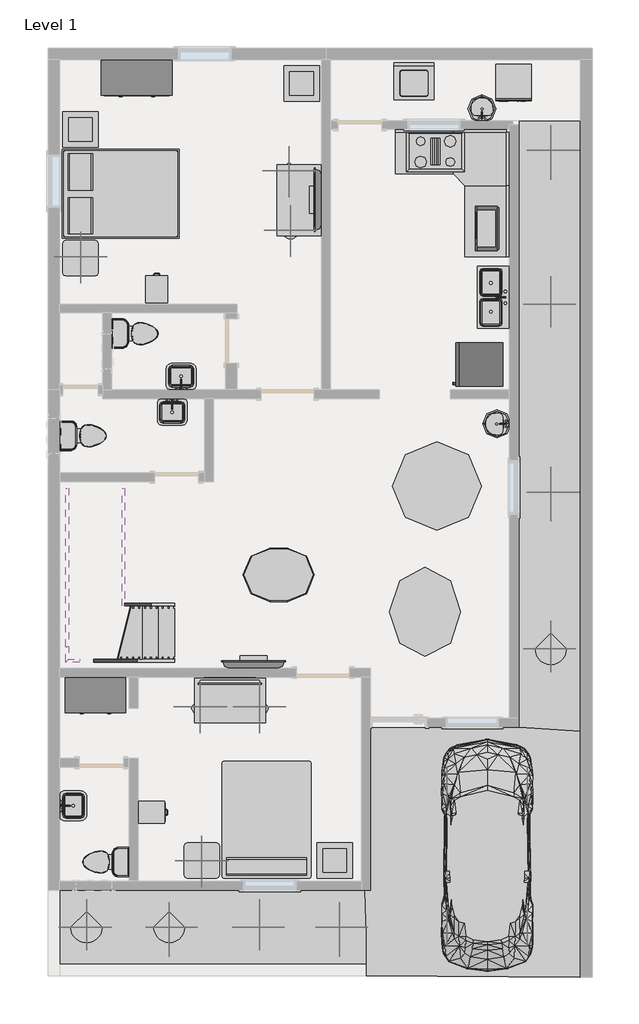
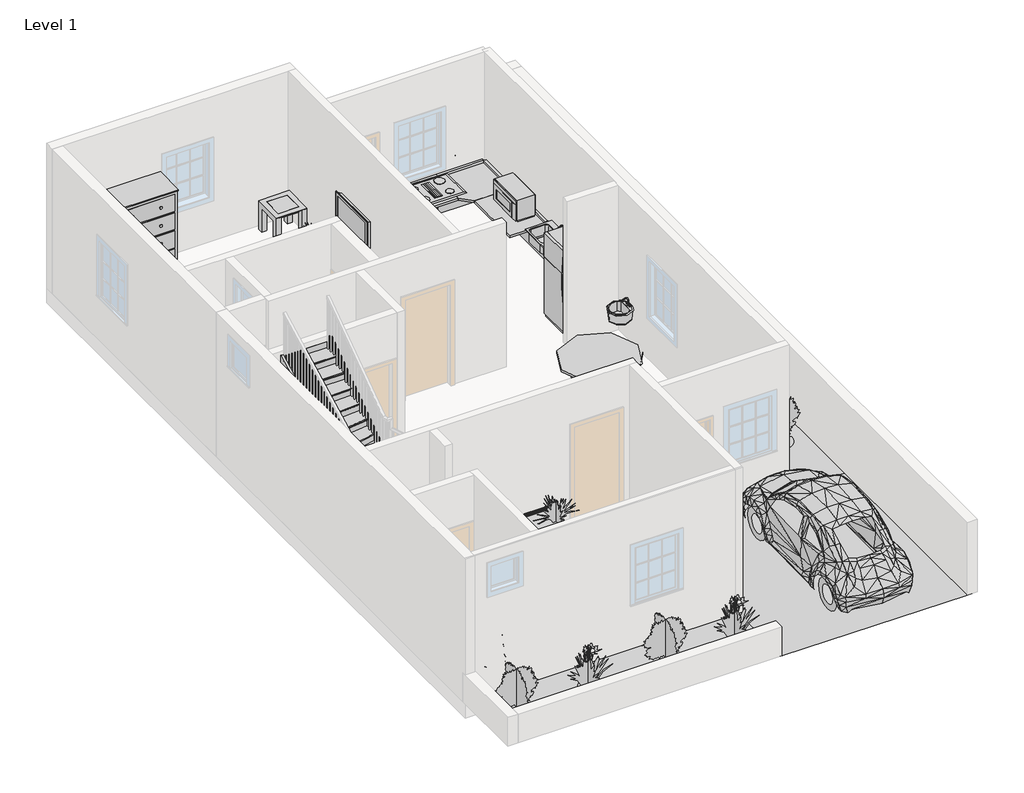
# One storey, part 3 of 3: 20 furniture elements, 14 geographic elements, 13 flow terminals, 9 proxies, 6 members, 1 stair flight.
"""IFC4 building model written with IfcOpenShell, lengths in millimetres."""

from ifc_helpers import new_model, si_unit, frame, origin, place, context, project, spatial, polyline, outline, extrude, triangles, transform, mapped, element, save
from components import proxy_bb1e6e30, proxy_45b28599, proxy_8a8d5ab2, rpc_beetle_rpc_beetle_3ce7ba48, proxy_a13a33b2, proxy_718fa39f, flow_terminal_accce45a, flow_terminal_a53be723, flow_terminal_d49f872f, flow_terminal_951b6bfb, flow_terminal_62a433f7, toilet_domestic_3d_toilet_domestic_3d_f7549cf7, toilet_domestic_3d_toilet_domestic_3d_183bbd19, furniture_1d2926bd, furniture_e1791683, furniture_bb55ed6b, furniture_9fa109b2, furniture_f72bdee3, furniture_7a3aaa4f, furniture_b5c51a22, furniture_be1c6672, furniture_bbcc68ce, furniture_743965d2, furniture_31d08a24, furniture_3f969c1c, furniture_5916b341, rpc_plant_tropical_55f6ff97, rpc_plant_tropical_agave_1_5_93a2a214, rpc_plant_tropical_jungle_flame_3_9c4808c2, stair_flight_28aaa101

model = new_model("IFC4")

# Units and contexts
model_context = context("Model", 3, world=origin())
ifc_project = project(units=[si_unit("LENGTHUNIT", "METRE", prefix="MILLI")], contexts=[model_context])

# Site, building, storey
site = spatial("IfcSite", under=ifc_project)
building = spatial("IfcBuilding", under=site)
storey = spatial("IfcBuildingStorey", under=building, Name="Level 1", Elevation=0.0)

# Proxies
placement = place(None, origin())
element("IfcBuildingElementProxy", 1, Name="Building Element Proxy", at=placement, inside=storey, context=model_context, shape_type="Tessellation", body=[
    triangles([(-6443.4660004, 13125.3534943, 0.0), (-5389.3658066, 13125.3534943, 0.0), (-5186.1660004, -971.6463604, 0.0), (-6433.8340302, -964.493018, 0.0)], [[1, 4, 2], [3, 2, 4]], closed=False),
])
element("IfcBuildingElementProxy", 2, Name="Building Element Proxy", at=placement, inside=storey, context=model_context, shape_type="Tessellation", body=[
    triangles([(-6443.4660004, 2711.353688, 0.0), (-9097.7661942, 2620.6554451, 0.0), (-9072.3660004, -147.5205558, 0.0), (-9096.8214844, -157.0514058, 0.0), (-9072.3660004, -1073.2463362, 0.0), (-6423.6154678, -976.648962, 0.0), (-9097.7661942, 2711.353688, 0.0), (-9072.3660004, -1555.846312, 0.0), (-5389.3658066, -1581.2463604, 0.0), (-5186.1660004, -1581.2463604, 0.0), (-5389.3658066, 2646.3030075, 0.0)], [[8, 5, 4], [5, 8, 6], [3, 2, 4], [7, 2, 1], [3, 4, 5], [6, 9, 10], [6, 3, 5], [6, 10, 11], [6, 1, 3], [1, 6, 11], [3, 1, 2], [6, 8, 9]], closed=False),
])
element("IfcBuildingElementProxy", 3, Name="Building Element Proxy", at=placement, inside=storey, context=model_context, shape_type="Tessellation", body=[
    triangles([(-14330.1660004, -82.6463725, 0.0), (-14330.1660004, -870.0463846, 0.0), (-9097.7661942, -82.6463725, 0.0), (-9072.3660004, -870.0463846, 0.0), (-14330.1660004, -1352.6463604, 0.0), (-9072.3660004, -1555.846312, 0.0)], [[4, 5, 6], [2, 5, 4], [1, 2, 3], [2, 4, 3]], closed=False),
])
proxy_shape = proxy_bb1e6e30(model_context)
element("IfcBuildingElementProxy", 4, Name="Cook Top-4 Unit : 36\" x 20\"", ObjectType="Cook Top-4 Unit : 36\" x 20\"", at=placement, inside=storey, context=model_context, shape_type="MappedRepresentation", body=[
    mapped(proxy_shape, transform((-7878.5660538, 12591.953629, 0.0), x_axis=(1.0, 0.0, 0.0), y_axis=(0.0, 1.0, 0.0), z_axis=(0.0, 0.0, 1.0))),
])
proxy_2_shape = proxy_45b28599(model_context)
element("IfcBuildingElementProxy", 5, Name="Dishwasher : 24\" x 24\" x 34\"", ObjectType="Dishwasher : 24\" x 24\" x 34\"", at=placement, inside=storey, context=model_context, shape_type="MappedRepresentation", body=[
    mapped(proxy_2_shape, transform((-6914.6835223, 13519.3040642, 0.0), x_axis=(1.0, 0.0, 0.0), y_axis=(0.0, 1.0, 0.0), z_axis=(0.0, 0.0, 1.0))),
])
proxy_3_shape = proxy_8a8d5ab2(model_context)
element("IfcBuildingElementProxy", 6, Name="Microwave : 30\" x 16\" x 18\"", ObjectType="Microwave : 30\" x 16\" x 18\"", at=placement, inside=storey, context=model_context, shape_type="MappedRepresentation", body=[
    mapped(proxy_3_shape, transform((-6636.485548, 11771.4465064, 0.0), x_axis=(0.0, -1.0000000000000007, 0.0), y_axis=(1.0000000000000007, 0.0, 0.0), z_axis=(0.0, 0.0, 1.0))),
])
rpc_beetle_rpc_beetle_shape = rpc_beetle_rpc_beetle_3ce7ba48(model_context)
element("IfcBuildingElementProxy", 7, Name="RPC Beetle : RPC Beetle", ObjectType="RPC Beetle : RPC Beetle", at=placement, inside=storey, context=model_context, shape_type="MappedRepresentation", body=[
    mapped(rpc_beetle_rpc_beetle_shape, transform((-6989.5660538, -717.646371, 0.0), x_axis=(1.0, 0.0, 0.0), y_axis=(0.0, 1.0, 0.0), z_axis=(0.0, 0.0, 1.0))),
])
proxy_4_shape = proxy_a13a33b2(model_context)
element("IfcBuildingElementProxy", 8, Name="Refrigerator : 30\" x 32\" RH", ObjectType="Refrigerator : 30\" x 32\" RH", at=placement, inside=storey, context=model_context, shape_type="MappedRepresentation", body=[
    mapped(proxy_4_shape, transform((-7109.0170823, 8942.291129, 0.0), x_axis=(0.0, -1.0000000000000007, 0.0), y_axis=(1.0000000000000007, 0.0, 0.0), z_axis=(0.0, 0.0, 1.0))),
])
proxy_5_shape = proxy_718fa39f(model_context)
element("IfcBuildingElementProxy", 9, Name="Washer : 27\" x 25\" x 35\"", ObjectType="Washer : 27\" x 25\" x 35\"", at=placement, inside=storey, context=model_context, shape_type="MappedRepresentation", body=[
    mapped(proxy_5_shape, transform((-8667.2835223, 13519.3040642, 0.0), x_axis=(1.0, 0.0, 0.0), y_axis=(0.0, 1.0, 0.0), z_axis=(0.0, 0.0, 1.0))),
])

# Flow terminals
flow_terminal_shape = flow_terminal_accce45a(model_context)
element("IfcFlowTerminal", 10, ObjectType="Floor Drain - Round : 5\" Strainer - 2\" Drain", at=placement, inside=storey, context=model_context, shape_type="MappedRepresentation", body=[
    mapped(flow_terminal_shape, transform((-13187.1660538, 8731.153629, 0.0), x_axis=(1.0, 0.0, 0.0), y_axis=(0.0, 1.0, 0.0), z_axis=(0.0, 0.0, 1.0))),
])
element("IfcFlowTerminal", 11, ObjectType="Floor Drain - Round : 5\" Strainer - 2\" Drain", at=placement, inside=storey, context=model_context, shape_type="MappedRepresentation", body=[
    mapped(flow_terminal_shape, transform((-13745.9660538, 7257.953629, 0.0), x_axis=(1.0, 0.0, 0.0), y_axis=(0.0, 1.0, 0.0), z_axis=(0.0, 0.0, 1.0))),
])
element("IfcFlowTerminal", 12, ObjectType="Floor Drain - Round : 5\" Strainer - 2\" Drain", at=placement, inside=storey, context=model_context, shape_type="MappedRepresentation", body=[
    mapped(flow_terminal_shape, transform((-14159.1367037, 774.6294473, 0.0), x_axis=(1.0, 0.0, 0.0), y_axis=(0.0, 1.0, 0.0), z_axis=(0.0, 0.0, 1.0))),
])
element("IfcFlowTerminal", 13, ObjectType="Floor Drain - Round : 5\" Strainer - 2\" Drain", at=placement, inside=storey, context=model_context, shape_type="MappedRepresentation", body=[
    mapped(flow_terminal_shape, transform((-7395.9660538, 13912.753629, 0.0), x_axis=(1.0, 0.0, 0.0), y_axis=(0.0, 1.0, 0.0), z_axis=(0.0, 0.0, 1.0))),
])
flow_terminal_2_shape = flow_terminal_a53be723(model_context)
element("IfcFlowTerminal", 14, ObjectType="Sink Kitchen-Double : 42\" x 21\"", at=placement, inside=storey, context=model_context, shape_type="MappedRepresentation", body=[
    mapped(flow_terminal_2_shape, transform((-6890.3114549, 10105.7428696, 0.0), x_axis=(0.0, -1.0000000000000002, 0.0), y_axis=(1.0000000000000002, 0.0, 0.0), z_axis=(0.0, 0.0, 1.0))),
])
flow_terminal_3_shape = flow_terminal_d49f872f(model_context)
element("IfcFlowTerminal", 15, ObjectType="Sink Vanity-Round : 19\" x 19\"", at=placement, inside=storey, context=model_context, shape_type="MappedRepresentation", body=[
    mapped(flow_terminal_3_shape, transform((-6981.8143133, 13408.8182168, 0.0), x_axis=(-1.0000000000000004, 0.0, 0.0), y_axis=(0.0, -1.0000000000000004, 0.0), z_axis=(0.0, 0.0, 1.0))),
])
flow_terminal_4_shape = flow_terminal_951b6bfb(model_context)
element("IfcFlowTerminal", 16, ObjectType="Sink Vanity-Round : 19\" x 19\"", at=placement, inside=storey, context=model_context, shape_type="MappedRepresentation", body=[
    mapped(flow_terminal_4_shape, transform((-6911.469597, 7821.7018885, 0.0), x_axis=(0.0, 1.0000000000000002, 0.0), y_axis=(-1.0000000000000002, 0.0, 0.0), z_axis=(0.0, 0.0, 1.0))),
])
flow_terminal_5_shape = flow_terminal_62a433f7(model_context)
element("IfcFlowTerminal", 17, ObjectType="Sink Vanity-Square : 20\" x 18\"", at=placement, inside=storey, context=model_context, shape_type="MappedRepresentation", body=[
    mapped(flow_terminal_5_shape, transform((-12231.6768133, 8682.6990301, 0.0), x_axis=(-1.0000000000000002, 0.0, 0.0), y_axis=(0.0, -1.0000000000000002, 0.0), z_axis=(0.0, 0.0, 1.0))),
])
element("IfcFlowTerminal", 18, ObjectType="Sink Vanity-Square : 20\" x 18\"", at=placement, inside=storey, context=model_context, shape_type="MappedRepresentation", body=[
    mapped(flow_terminal_5_shape, transform((-12415.4552944, 8170.0082279, 0.0), x_axis=(1.0, 0.0, 0.0), y_axis=(0.0, 1.0, 0.0), z_axis=(0.0, 0.0, 1.0))),
])
element("IfcFlowTerminal", 19, ObjectType="Sink Vanity-Square : 20\" x 18\"", at=placement, inside=storey, context=model_context, shape_type="MappedRepresentation", body=[
    mapped(flow_terminal_5_shape, transform((-14150.0206527, 1349.4643885, 0.0), x_axis=(0.0, 1.0000000000000002, 0.0), y_axis=(-1.0000000000000002, 0.0, 0.0), z_axis=(0.0, 0.0, 1.0))),
])
toilet_domestic_3d_toilet_domestic_3d_shape = toilet_domestic_3d_toilet_domestic_3d_f7549cf7(model_context)
toilet_domestic_3d_toilet_domestic_3d_2_shape = toilet_domestic_3d_toilet_domestic_3d_183bbd19(model_context)
element("IfcFlowTerminal", 20, ObjectType="Toilet-Domestic-3D : Toilet-Domestic-3D", at=placement, inside=storey, context=model_context, shape_type="MappedRepresentation", body=[
    mapped(toilet_domestic_3d_toilet_domestic_3d_shape, transform((-12946.4700265, 9467.753629, 0.0), x_axis=(0.0, 1.0, 0.0), y_axis=(-1.0, 0.0, 0.0), z_axis=(0.0, 0.0, 1.0))),
    mapped(toilet_domestic_3d_toilet_domestic_3d_2_shape, transform((-12946.4700265, 9467.753629, 0.0), x_axis=(0.0, 1.0, 0.0), y_axis=(-1.0, 0.0, 0.0), z_axis=(0.0, 0.0, 1.0))),
])
element("IfcFlowTerminal", 21, ObjectType="Toilet-Domestic-3D : Toilet-Domestic-3D", at=placement, inside=storey, context=model_context, shape_type="MappedRepresentation", body=[
    mapped(toilet_domestic_3d_toilet_domestic_3d_shape, transform((-13835.4700265, 7715.153629, 0.0), x_axis=(0.0, 1.0, 0.0), y_axis=(-1.0, 0.0, 0.0), z_axis=(0.0, 0.0, 1.0))),
    mapped(toilet_domestic_3d_toilet_domestic_3d_2_shape, transform((-13835.4700265, 7715.153629, 0.0), x_axis=(0.0, 1.0, 0.0), y_axis=(-1.0, 0.0, 0.0), z_axis=(0.0, 0.0, 1.0))),
])
element("IfcFlowTerminal", 22, ObjectType="Toilet-Domestic-3D : Toilet-Domestic-3D", at=placement, inside=storey, context=model_context, shape_type="MappedRepresentation", body=[
    mapped(toilet_domestic_3d_toilet_domestic_3d_shape, transform((-13631.0620812, 399.953629, 0.0), x_axis=(0.0, -1.0000000000000004, 0.0), y_axis=(1.0000000000000004, 0.0, 0.0), z_axis=(0.0, 0.0, 1.0))),
    mapped(toilet_domestic_3d_toilet_domestic_3d_2_shape, transform((-13631.0620812, 399.953629, 0.0), x_axis=(0.0, -1.0000000000000004, 0.0), y_axis=(1.0000000000000004, 0.0, 0.0), z_axis=(0.0, 0.0, 1.0))),
])

# Furniture
furniture_shape = furniture_1d2926bd(model_context)
element("IfcFurniture", 23, ObjectType="Bed-Box : Queen 60\" x 79\"", at=placement, inside=storey, context=model_context, shape_type="MappedRepresentation", body=[
    mapped(furniture_shape, transform((-13517.3660538, 11528.90117, 0.0), x_axis=(0.0, 1.0, 0.0), y_axis=(-1.0, 0.0, 0.0), z_axis=(0.0, 0.0, 1.0))),
])
furniture_2_shape = furniture_e1791683(model_context)
element("IfcFurniture", 24, ObjectType="Bed-Standard.0001 : Queen 60\" x 79\"", at=placement, inside=storey, context=model_context, shape_type="MappedRepresentation", body=[
    mapped(furniture_2_shape, transform((-10509.0275292, 1078.2585471, 0.0), x_axis=(-1.0, 0.0, 0.0), y_axis=(0.0, -1.0, 0.0), z_axis=(0.0, 0.0, 1.0))),
])
furniture_3_shape = furniture_bb55ed6b(model_context)
element("IfcFurniture", 25, ObjectType="Cabinet-File 2 Drawer : 15\" x 18\"", at=placement, inside=storey, context=model_context, shape_type="MappedRepresentation", body=[
    mapped(furniture_3_shape, transform((-12794.3625009, 10087.6193289, 0.0), x_axis=(-0.9999999999999999, 0.0, 0.0), y_axis=(0.0, -0.9999999999999999, 0.0), z_axis=(0.0, 0.0, 1.0))),
])
element("IfcFurniture", 26, ObjectType="Cabinet-File 2 Drawer : 15\" x 18\"", at=placement, inside=storey, context=model_context, shape_type="MappedRepresentation", body=[
    mapped(furniture_3_shape, transform((-12897.5003539, 1379.8516209, 0.0), x_axis=(0.0, 1.0, 0.0), y_axis=(-1.0, 0.0, 0.0), z_axis=(0.0, 0.0, 1.0))),
])
furniture_4_shape = furniture_9fa109b2(model_context)
element("IfcFurniture", 27, ObjectType="Dresser : 48\" x 72\" x 24\"", at=placement, inside=storey, context=model_context, shape_type="MappedRepresentation", body=[
    mapped(furniture_4_shape, transform((-12740.172794, 14225.1165831, 0.0), x_axis=(1.0, 0.0, 0.0), y_axis=(0.0, 1.0, 0.0), z_axis=(0.0, 0.0, 1.0))),
])
furniture_5_shape = furniture_f72bdee3(model_context)
element("IfcFurniture", 28, ObjectType="Dresser : 48\" x 72\" x 24\" 2", at=placement, inside=storey, context=model_context, shape_type="MappedRepresentation", body=[
    mapped(furniture_5_shape, transform((-13451.372794, 3633.3165831, 0.0), x_axis=(1.0, 0.0, 0.0), y_axis=(0.0, 1.0, 0.0), z_axis=(0.0, 0.0, 1.0))),
])
furniture_6_shape = furniture_7a3aaa4f(model_context)
element("IfcFurniture", 29, ObjectType="TV - Flat Screen : 42\"", at=placement, inside=storey, context=model_context, shape_type="MappedRepresentation", body=[
    mapped(furniture_6_shape, transform((-9892.9046775, 11762.5091149, 990.6), x_axis=(0.0, -1.0000000000000002, 0.0), y_axis=(1.0000000000000002, 0.0, 0.0), z_axis=(0.0, 0.0, 1.0))),
])
element("IfcFurniture", 30, ObjectType="TV - Flat Screen : 42\"", at=placement, inside=storey, context=model_context, shape_type="MappedRepresentation", body=[
    mapped(furniture_6_shape, transform((-11405.2215397, 3516.4150054, 0.0), x_axis=(1.0, 0.0, 0.0), y_axis=(0.0, 1.0, 0.0), z_axis=(0.0, 0.0, 1.0))),
])
element("IfcFurniture", 31, ObjectType="TV - Flat Screen : 42\"", at=placement, inside=storey, context=model_context, shape_type="MappedRepresentation", body=[
    mapped(furniture_6_shape, transform((-11006.710568, 3785.8922527, 990.6), x_axis=(-1.0000000000000002, 0.0, 0.0), y_axis=(0.0, -1.0000000000000002, 0.0), z_axis=(0.0, 0.0, 1.0))),
])
furniture_7_shape = furniture_b5c51a22(model_context)
element("IfcFurniture", 32, ObjectType="Table-Coffee : 24\" x 24\" x 24\"", at=placement, inside=storey, context=model_context, shape_type="MappedRepresentation", body=[
    mapped(furniture_7_shape, transform((-13992.8318205, 12877.7425512, 0.0), x_axis=(1.0, 0.0, 0.0), y_axis=(0.0, 1.0, 0.0), z_axis=(0.0, 0.0, 1.0))),
])
element("IfcFurniture", 33, ObjectType="Table-Coffee : 24\" x 24\" x 24\"", at=placement, inside=storey, context=model_context, shape_type="MappedRepresentation", body=[
    mapped(furniture_7_shape, transform((-10195.5318205, 13665.1425512, 0.0), x_axis=(1.0, 0.0, 0.0), y_axis=(0.0, 1.0, 0.0), z_axis=(0.0, 0.0, 1.0))),
])
element("IfcFurniture", 34, ObjectType="Table-Coffee : 24\" x 24\" x 24\"", at=placement, inside=storey, context=model_context, shape_type="MappedRepresentation", body=[
    mapped(furniture_7_shape, transform((-9624.0318205, 330.1425512, 0.0), x_axis=(1.0, 0.0, 0.0), y_axis=(0.0, 1.0, 0.0), z_axis=(0.0, 0.0, 1.0))),
])
furniture_8_shape = furniture_be1c6672(model_context)
element("IfcFurniture", 35, ObjectType="Table-Dining Oval : 36\" x 48\"", at=placement, inside=storey, context=model_context, shape_type="MappedRepresentation", body=[
    mapped(furniture_8_shape, transform((-10169.1463817, 5685.6519897, 0.0), x_axis=(1.0, 0.0, 0.0), y_axis=(0.0, 1.0, 0.0), z_axis=(0.0, 0.0, 1.0))),
])
furniture_9_shape = furniture_bbcc68ce(model_context)
element("IfcFurniture", 36, ObjectType="Table-Dining Round w Chairs : 60\" Diameter", at=placement, inside=storey, context=model_context, shape_type="MappedRepresentation", body=[
    mapped(furniture_9_shape, transform((-7956.848021, 7036.4323176, 0.0), x_axis=(1.0, 0.0, 0.0), y_axis=(0.0, 1.0, 0.0), z_axis=(0.0, 0.0, 1.0))),
])
furniture_10_shape = furniture_743965d2(model_context)
element("IfcFurniture", 37, ObjectType="Table-Ellipse : 60\" x 48\"", at=placement, inside=storey, context=model_context, shape_type="MappedRepresentation", body=[
    mapped(furniture_10_shape, transform((-8056.3660538, 4692.553629, 0.0), x_axis=(0.0, 1.0000000000000002, 0.0), y_axis=(-1.0000000000000002, 0.0, 0.0), z_axis=(0.0, 0.0, 1.0))),
])
furniture_11_shape = furniture_31d08a24(model_context)
element("IfcFurniture", 38, ObjectType="Table-End : 24\" x 24\"", at=placement, inside=storey, context=model_context, shape_type="MappedRepresentation", body=[
    mapped(furniture_11_shape, transform((-14283.0996841, 10610.753629, 0.0), x_axis=(1.0, 0.0, 0.0), y_axis=(0.0, 1.0, 0.0), z_axis=(0.0, 0.0, 1.0))),
])
element("IfcFurniture", 39, ObjectType="Table-End : 24\" x 24\"", at=placement, inside=storey, context=model_context, shape_type="MappedRepresentation", body=[
    mapped(furniture_11_shape, transform((-12200.2996841, 272.953629, 0.0), x_axis=(1.0, 0.0, 0.0), y_axis=(0.0, 1.0, 0.0), z_axis=(0.0, 0.0, 1.0))),
])
furniture_12_shape = furniture_3f969c1c(model_context)
element("IfcFurniture", 40, ObjectType="Table-Rectangular : 72\" x 30\"", at=placement, inside=storey, context=model_context, shape_type="MappedRepresentation", body=[
    mapped(furniture_12_shape, transform((-10215.3660538, 11753.753629, 0.0), x_axis=(0.0, 1.0000000000000002, 0.0), y_axis=(-1.0000000000000002, 0.0, 0.0), z_axis=(0.0, 0.0, 1.0))),
])
element("IfcFurniture", 41, ObjectType="Table-Rectangular : 72\" x 30\"", at=placement, inside=storey, context=model_context, shape_type="MappedRepresentation", body=[
    mapped(furniture_12_shape, transform((-11409.1660538, 3168.553629, 0.0), x_axis=(1.0, 0.0, 0.0), y_axis=(0.0, 1.0, 0.0), z_axis=(0.0, 0.0, 1.0))),
])
furniture_13_shape = furniture_5916b341(model_context)
element("IfcFurniture", 42, ObjectType="Work Station Cubicle : 96\" x 96\"", at=placement, inside=storey, context=model_context, shape_type="MappedRepresentation", body=[
    mapped(furniture_13_shape, transform((-6113.5430462, 12841.2218768, 0.0), x_axis=(0.0, -1.0000000000000004, 0.0), y_axis=(1.0000000000000004, 0.0, 0.0), z_axis=(0.0, 0.0, 1.0))),
])

# Geographic elements
rpc_plant_tropical_shape = rpc_plant_tropical_55f6ff97(model_context)
element("IfcGeographicElement", 43, ObjectType="RPC Plant - Tropical", at=placement, inside=storey, context=model_context, shape_type="MappedRepresentation", body=[
    mapped(rpc_plant_tropical_shape, transform((-5897.3660538, 12617.353629, 0.0), x_axis=(1.0, 0.0, 0.0), y_axis=(0.0, 1.0, 0.0), z_axis=(0.0, 0.0, 1.0))),
])
element("IfcGeographicElement", 44, ObjectType="RPC Plant - Tropical", at=placement, inside=storey, context=model_context, shape_type="MappedRepresentation", body=[
    mapped(rpc_plant_tropical_shape, transform((-5897.3660538, 6749.953629, 0.0), x_axis=(1.0, 0.0, 0.0), y_axis=(0.0, 1.0, 0.0), z_axis=(0.0, 0.0, 1.0))),
])
element("IfcGeographicElement", 45, ObjectType="RPC Plant - Tropical", at=placement, inside=storey, context=model_context, shape_type="MappedRepresentation", body=[
    mapped(rpc_plant_tropical_shape, transform((-12450.5660538, -717.646371, 0.0), x_axis=(1.0, 0.0, 0.0), y_axis=(0.0, 1.0, 0.0), z_axis=(0.0, 0.0, 1.0))),
])
element("IfcGeographicElement", 46, ObjectType="RPC Plant - Tropical", at=placement, inside=storey, context=model_context, shape_type="MappedRepresentation", body=[
    mapped(rpc_plant_tropical_shape, transform((-9529.5660538, -717.646371, 0.0), x_axis=(1.0, 0.0, 0.0), y_axis=(0.0, 1.0, 0.0), z_axis=(0.0, 0.0, 1.0))),
])
rpc_plant_tropical_agave_1_5_shape = rpc_plant_tropical_agave_1_5_93a2a214(model_context)
element("IfcGeographicElement", 47, ObjectType="RPC Plant - Tropical : Agave - 1.5'", at=placement, inside=storey, context=model_context, shape_type="MappedRepresentation", body=[
    mapped(rpc_plant_tropical_agave_1_5_shape, transform((-13974.5660538, 10788.553629, 609.6), x_axis=(1.0, 0.0, 0.0), y_axis=(0.0, 1.0, 0.0), z_axis=(0.0, 0.0, 1.0))),
])
element("IfcGeographicElement", 48, ObjectType="RPC Plant - Tropical : Agave - 1.5'", at=placement, inside=storey, context=model_context, shape_type="MappedRepresentation", body=[
    mapped(rpc_plant_tropical_agave_1_5_shape, transform((-10393.1660538, 12261.753629, 660.4), x_axis=(1.0, 0.0, 0.0), y_axis=(0.0, 1.0, 0.0), z_axis=(0.0, 0.0, 1.0))),
])
element("IfcGeographicElement", 49, ObjectType="RPC Plant - Tropical : Agave - 1.5'", at=placement, inside=storey, context=model_context, shape_type="MappedRepresentation", body=[
    mapped(rpc_plant_tropical_agave_1_5_shape, transform((-10367.7660538, 11245.753629, 660.4), x_axis=(1.0, 0.0, 0.0), y_axis=(0.0, 1.0, 0.0), z_axis=(0.0, 0.0, 1.0))),
])
element("IfcGeographicElement", 50, ObjectType="RPC Plant - Tropical : Agave - 1.5'", at=placement, inside=storey, context=model_context, shape_type="MappedRepresentation", body=[
    mapped(rpc_plant_tropical_agave_1_5_shape, transform((-11891.7660538, 425.353629, 609.6), x_axis=(1.0, 0.0, 0.0), y_axis=(0.0, 1.0, 0.0), z_axis=(0.0, 0.0, 1.0))),
])
element("IfcGeographicElement", 51, ObjectType="RPC Plant - Tropical : Agave - 1.5'", at=placement, inside=storey, context=model_context, shape_type="MappedRepresentation", body=[
    mapped(rpc_plant_tropical_agave_1_5_shape, transform((-11917.1660538, 3066.953629, 660.4), x_axis=(1.0, 0.0, 0.0), y_axis=(0.0, 1.0, 0.0), z_axis=(0.0, 0.0, 1.0))),
])
element("IfcGeographicElement", 52, ObjectType="RPC Plant - Tropical : Agave - 1.5'", at=placement, inside=storey, context=model_context, shape_type="MappedRepresentation", body=[
    mapped(rpc_plant_tropical_agave_1_5_shape, transform((-10901.1660538, 3066.953629, 660.4), x_axis=(1.0, 0.0, 0.0), y_axis=(0.0, 1.0, 0.0), z_axis=(0.0, 0.0, 1.0))),
])
rpc_plant_tropical_jungle_flame_3_shape = rpc_plant_tropical_jungle_flame_3_9c4808c2(model_context)
element("IfcGeographicElement", 53, ObjectType="RPC Plant - Tropical : Jungle Flame - 3'", at=placement, inside=storey, context=model_context, shape_type="MappedRepresentation", body=[
    mapped(rpc_plant_tropical_jungle_flame_3_shape, transform((-5897.3660538, 9975.753629, 0.0), x_axis=(1.0, 0.0, 0.0), y_axis=(0.0, 1.0, 0.0), z_axis=(0.0, 0.0, 1.0))),
])
element("IfcGeographicElement", 54, ObjectType="RPC Plant - Tropical : Jungle Flame - 3'", at=placement, inside=storey, context=model_context, shape_type="MappedRepresentation", body=[
    mapped(rpc_plant_tropical_jungle_flame_3_shape, transform((-5897.3660538, 4057.553629, 0.0), x_axis=(1.0, 0.0, 0.0), y_axis=(0.0, 1.0, 0.0), z_axis=(0.0, 0.0, 1.0))),
])
element("IfcGeographicElement", 55, ObjectType="RPC Plant - Tropical : Jungle Flame - 3'", at=placement, inside=storey, context=model_context, shape_type="MappedRepresentation", body=[
    mapped(rpc_plant_tropical_jungle_flame_3_shape, transform((-13872.9660538, -717.646371, 0.0), x_axis=(1.0, 0.0, 0.0), y_axis=(0.0, 1.0, 0.0), z_axis=(0.0, 0.0, 1.0))),
])
element("IfcGeographicElement", 56, ObjectType="RPC Plant - Tropical : Jungle Flame - 3'", at=placement, inside=storey, context=model_context, shape_type="MappedRepresentation", body=[
    mapped(rpc_plant_tropical_jungle_flame_3_shape, transform((-10901.1660538, -717.646371, 0.0), x_axis=(1.0, 0.0, 0.0), y_axis=(0.0, 1.0, 0.0), z_axis=(0.0, 0.0, 1.0))),
])

# Members
element("IfcMember", 57, ObjectType="Stringer - 2\" Width", at=placement, inside=storey, context=model_context, shape_type="SweptSolid", body=[
    extrude(outline(polyline([(590.0562463, -12359.4290643), (922.8849999, -12359.4290643), (1638.0971411, -13990.0912571), (1305.2683876, -13990.0912571), (590.0562463, -12359.4290643)])), frame((0.0, 3828.953629, 0.0), z_axis=(0.0, 1.0, 0.0), x_axis=(0.0, 0.0, 1.0)), (0.0, 0.0, 1.0), 50.8),
])
element("IfcMember", 58, ObjectType="Stringer - 2\" Width", at=placement, inside=storey, context=model_context, shape_type="SweptSolid", body=[
    extrude(outline(polyline([(-13990.0912571, 3879.753629), (-13990.0912571, 3828.953629), (-14228.5660538, 3828.953629), (-14177.7660538, 3879.753629), (-13990.0912571, 3879.753629)])), frame((0.0, 0.0, 1305.2683876), z_axis=(0.0, 0.0, 1.0), x_axis=(1.0, 0.0, 0.0)), (0.0, 0.0, 1.0), 332.8287535),
])
element("IfcMember", 59, ObjectType="Stringer - 2\" Width", at=placement, inside=storey, context=model_context, shape_type="SweptSolid", body=[
    extrude(outline(polyline([(-14177.7660538, 3879.753629), (-14228.5660538, 3828.953629), (-14228.5660538, 4097.9069721), (-14177.7660538, 4097.9069721), (-14177.7660538, 3879.753629)])), frame((0.0, 0.0, 1305.2683876), z_axis=(0.0, 0.0, 1.0), x_axis=(1.0, 0.0, 0.0)), (0.0, 0.0, 1.0), 332.8287535),
])
element("IfcMember", 60, ObjectType="Stringer - 2\" Width", at=placement, inside=storey, context=model_context, shape_type="SweptSolid", body=[
    extrude(outline(polyline([(4097.9069721, 1305.2683876), (4097.9069721, 1638.0971411), (6815.6906185, 3053.6189504), (6815.6906185, 2720.7901969), (4097.9069721, 1305.2683876)])), frame((-14228.5660538, 0.0, 0.0), z_axis=(1.0, 0.0, 0.0), x_axis=(0.0, 1.0, 0.0)), (0.0, 0.0, 1.0), 50.8),
])
element("IfcMember", 61, ObjectType="Stringer - 2\" Width", at=placement, inside=storey, context=model_context, shape_type="SweptSolid", body=[
    extrude(outline(polyline([(435.4922729, -12359.4290643), (842.634734, -12359.4290643), (1598.1690344, -13212.5660538), (1191.0265733, -13212.5660538), (435.4922729, -12359.4290643)])), frame((0.0, 4794.153629, 0.0), z_axis=(0.0, 1.0, 0.0), x_axis=(0.0, 0.0, 1.0)), (0.0, 0.0, 1.0), 50.8),
])
element("IfcMember", 62, ObjectType="Stringer - 2\" Width", at=placement, inside=storey, context=model_context, shape_type="SweptSolid", body=[
    extrude(outline(polyline([(4794.153629, 1337.7212805), (4794.153629, 1709.9296678), (6815.6906185, 3126.7693854), (6815.6906185, 2754.5609981), (4794.153629, 1337.7212805)])), frame((-13263.3660538, 0.0, 0.0), z_axis=(1.0, 0.0, 0.0), x_axis=(0.0, 1.0, 0.0)), (0.0, 0.0, 1.0), 50.8),
])

# Stair flight
stair_flight_shape = stair_flight_28aaa101(model_context)
element("IfcStairFlight", 63, ObjectType="2\" Tread 1\" Nosing 1/4\" Riser", at=placement, inside=storey, context=model_context, shape_type="MappedRepresentation", body=[
    mapped(stair_flight_shape, transform((0.0, 0.0, 0.0), x_axis=(1.0, 0.0, 0.0), y_axis=(0.0, 1.0, 0.0), z_axis=(0.0, 0.0, 1.0))),
])

save(model, "model.ifc")

# Revit data of these elements
# Type "Cook Top-4 Unit : 36\" x 20\""
#   Assembly Code = "E1090400"
#   Depth = 2' - 0"
#   Width = 3' - 0"
#   Burner Material = Steel, Chrome Plated
#   Cooktop Material = Steel, Polished
#   Default Elevation = 0
# Type "Dishwasher : 24\" x 24\" x 34\""
#   Label = "DW"
#   Assembly Code = "E1090400"
#   Depth = 2' - 0"
#   Height = 2' - 10"
#   Width = 2' - 0"
#   Dishwasher Material = Steel, Paint Finish, Ivory, Glossy
#   Panel Face Material = Plastic, Opaque Black
#   Default Elevation = 0
# Type "Microwave : 30\" x 16\" x 18\""
#   Assembly Code = "E1090400"
#   Depth = 1' - 4"
#   Height = 1' - 6"
#   Width = 2' - 6"
#   Microwave Material = Laminate, Ivory, Matte
#   Default Elevation = 0
# Type "RPC Beetle : RPC Beetle"
#   built-in parameter 1005195 = "RPC-16-0U6E-L4EG-ENH1-J3KF-SVEL-0TX4-C0"
#   Height = 0
# Type "Refrigerator : 30\" x 32\" RH"
#   Label = "REF."
#   Assembly Code = "E1090400"
#   Depth = 2' - 7 3/4"
#   Handle = 2' - 3"
#   Height = 5' - 10"
#   Rear Clearance = 0' - 2"
#   Top Door Height = 1' - 8"
#   Width = 2' - 5 3/8"
#   Material = Steel, Paint Finish, Ivory, Glossy
#   Default Elevation = 0
# Type "Washer : 27\" x 25\" x 35\""
#   Label = "W"
#   Assembly Code = "E1090400"
#   Depth = 2' - 1"
#   Height = 2' - 11"
#   Width = 2' - 3"
#   Washer Material = Steel, Paint Finish, Ivory, Matte
#   Default Elevation = 0
# Type "Floor Drain - Round : 5\" Strainer - 2\" Drain"
#   WFU = 2
#   Strainer Height = 0' - 3 1/4"
#   Strainer Radius = 0' - 2 1/2"
#   Strainer Diameter = 0' - 5"
#   Radius 6 = 0' - 0 5/8"
#   Radius 5 = 0' - 1 1/4"
#   Radius 4 = 0' - 1 7/8"
#   Radius 2 = 0' - 3.04167"
#   Radius 1 = 0' - 2.02083"
#   Radius 3 = 0' - 2 1/32"
#   Pipe Radius = 1"
#   Pipe Diameter = 2"
#   Height 2 = 0' - 0.725"
#   Height 1 = 0' - 1 13/16"
#   Body Radius = 0' - 4 1/16"
#   Body Height = 0' - 3 5/8"
#   Body Diameter = 0' - 8 1/8"
#   Drain Material = none
#   HWFU = 0
#   Default Elevation = 0
#   CWFU = 0
# Type "Sink Kitchen-Double : 42\" x 21\""
#   Assembly Code = "D2010410"
#   Counter Height = 3' - 0"
#   Depth = 1' - 9"
#   Width = 3' - 6"
#   Faucet Material = Steel, Polished
#   Sink Material = Steel, Polished
#   Default Elevation = 0
# Type "Sink Vanity-Round : 19\" x 19\""
#   Assembly Code = "D2010400"
#   Top Of Counter = 2' - 7"
#   Basin Material = Porcelain, Linen
#   Faucet Material = Steel, Polished
#   Default Elevation = 0
# Type "Sink Vanity-Square : 20\" x 18\""
#   Assembly Code = "D2010400"
#   Counter Height = 2' - 7"
#   Depth = 1' - 6"
#   Width = 1' - 8"
#   Basin Material = Porcelain, Linen
#   Faucet Material = Steel, Polished
#   Default Elevation = 0
# Type "Toilet-Domestic-3D : Toilet-Domestic-3D"
#   Assembly Code = "D2010110"
#   Toilet - Bowl/Basin Material = Porcelain, Linen
#   Toilet - Seat Material = Laminate, Linen, Matte
#   Default Elevation = 0
# Type "Bed-Box : Queen 60\" x 79\""
#   Assembly Code = "E2020200"
#   Length = 6' - 7"
#   Width = 5' - 0"
#   Frame Material = Birch
#   Mattress Material = Sash
#   Default Elevation = 0
# Type "Bed-Standard.0001 : Queen 60\" x 79\""
#   Assembly Code = "E2020200"
#   Length = 6' - 7"
#   Width = 5' - 0"
#   Leg Material = Steel, Chrome Plated
#   Mattress Material = Linen, White
#   Default Elevation = 0
# Type "Cabinet-File 2 Drawer : 15\" x 18\""
#   Assembly Code = "E2020200"
#   Depth = 1' - 6"
#   Height = 2' - 5"
#   Width = 1' - 3"
#   Cabinet Material = Steel, Paint Finish, Ivory, Glossy
#   Handle Material = Steel, Chrome Plated
#   Default Elevation = 0
# Type "Dresser : 48\" x 72\" x 24\""
#   Assembly Code = "E2020200"
#   Depth = 2' - 0"
#   Height = 6' - 0"
#   Width = 4' - 0"
#   Dresser Material = Wood - Teak
#   Drawer Material = Wood - Teak
#   Knob Material = Cherry
#   Default Elevation = 0
# Type "Dresser : 48\" x 72\" x 24\" 2"
#   Assembly Code = "E2020200"
#   Depth = 2' - 0"
#   Height = 6' - 0"
#   Width = 3' - 5"
#   Dresser Material = Wood - Teak
#   Drawer Material = Wood - Teak
#   Knob Material = Cherry
#   Default Elevation = 0
# Type "TV - Flat Screen : 42\""
#   SinAng = 0' - 0.0193"
#   L = 3' - 0.71517"
#   H = 1' - 8.65418"
#   Thickness = 0' - 4.33071"
#   Diagonal = 3' - 6.12598"
#   CosAng = 0' - 0.03431"
#   Stand [instance default] = yes
#   Default Elevation = 0
# Type "Table-Coffee : 24\" x 24\" x 24\""
#   Assembly Code = "E2020200"
#   Height = 2' - 0"
#   Length = 2' - 0"
#   Width = 2' - 0"
#   Top Material = none
#   Frame Material = none
#   Default Elevation = 0
# Type "Table-Dining Oval : 36\" x 48\""
#   Assembly Code = "E2020200"
#   Length = 4' - 0"
#   Width = 3' - 0"
#   Base Material = Steel, Chrome Plated
#   Top Material = Glass - Clear, Grey
#   Default Elevation = 0
#   Description = (empty or 0)
# Type "Table-Dining Round w Chairs : 60\" Diameter"
#   Assembly Code = "E2020200"
#   Radius = 2' - 6"
#   Diameter = 5' - 0"
#   Height = 2' - 6"
#   Chairs = 6
#   Base Material = Pine
#   Top Material = Laminate, Linen, Matte
#   Default Elevation = 0
# Type "Table-Ellipse : 60\" x 48\""
#   Assembly Code = "E2020200"
#   Half Width = 2' - 0"
#   Half Length = 2' - 6"
#   Height = 2' - 6"
#   Length = 5' - 0"
#   Width = 4' - 0"
#   Base Material = Birch
#   Top Material = Birch
#   Default Elevation = 0
# Type "Table-End : 24\" x 24\""
#   Assembly Code = "E2020200"
#   Height = 2' - 0"
#   Length = 2' - 0"
#   Width = 2' - 0"
#   Base Material = Birch
#   Top Material = Laminate, Ivory, Matte
#   Default Elevation = 0
# Type "Table-Rectangular : 72\" x 30\""
#   Assembly Code = "E2020200"
#   Height = 2' - 2"
#   Length = 4' - 0"
#   Width = 2' - 6"
#   Base Material = Birch
#   Top Material = Birch
#   Default Elevation = 0
# Type "Work Station Cubicle : 96\" x 96\""
#   Assembly Code = "E2020"
#   Desktop Height = 2' - 6"
#   Desktop1 Width = 2' - 4"
#   Desktop2 Width = 2' - 4"
#   Panel Height = 2' - 8"
#   Panel1 Length = 3' - 3"
#   Panel2 Length = 4' - 0"
#   Cube Panel Material = Textile - Light Gray
#   Work Top Material = Laminate, Ivory, Matte
#   Default Elevation = 0
# Type "RPC Plant - Tropical"
#   built-in parameter 1005198 = "{2, 15},{39, RPC-16-FWM5-GM7X-C67P-4000-ST1L-LVER-AU},{1, 0},{1, 0},{2, 13},{1, 8},{5, Color},{1, 0},{1, 0},{3, 0.8},{3, 0.8},{3, 0.8},{1, 8},{7, BBoxMin},{1, 0},{1, 0},{1, 0},{1, 0},{1, 0},{1, 8},{7, BBoxMax},{1, 0},{1, 0},{1, 0},{1, 0},{1, 0},{2, 11},{9, RPCTypeId},{1, 0},{1, 0},{39, RPC-16-FWM5-GM7X-C67P-4000-ST1L-LVER-AU},{1, 6},{14, RPCPlantHeight},{1, 0},{1, 0},{1, 3},{2, 11},{7, keyword},{1, 0},{1, 0},{35, :RPCs:Shrubs [General]:Geometry:RPC},{2, 11},{8, category},{1, 0},{1, 0},{16, Shrubs [General]},{2, 11},{12, LocalizedUID},{1, 0},{1, 0},{10, Crane Lily},{2, 14},{6, Height},{1, 0},{1, 0},{1, 3},{1, 2},{16, Cast Reflections},{1, 0},{1, 0},{1, 0},{1, 2},{12, Cast Shadows},{1, 0},{1, 0},{1, 1},{1, 2},{9, Lock View},{1, 0},{1, 0},{1, 0},{1, 4},{5, ViewC},{1, 0},{1, 0},{1, 0},{21, assetlibrary_base.fbx},{1, 5},"
#   built-in parameter 1005195 = "RPC-16-FWM5-GM7X-C67P-4000-ST1L-LVER-AU"
#   Assembly Code = "G2050500"
#   Height = 3' - 0"
#   Default Elevation = 0
# Type "RPC Plant - Tropical : Agave - 1.5'"
#   built-in parameter 1005198 = "{2, 15},{39, RPC-16-G1GJ-63FX-7K5P-N000-ST1L-LVER-AU},{1, 0},{1, 0},{2, 13},{1, 8},{5, Color},{1, 0},{1, 0},{3, 0.8},{3, 0.8},{3, 0.8},{1, 8},{7, BBoxMin},{1, 0},{1, 0},{1, 0},{1, 0},{1, 0},{1, 8},{7, BBoxMax},{1, 0},{1, 0},{1, 0},{1, 0},{1, 0},{2, 11},{9, RPCTypeId},{1, 0},{1, 0},{39, RPC-16-G1GJ-63FX-7K5P-N000-ST1L-LVER-AU},{1, 6},{14, RPCPlantHeight},{1, 0},{1, 0},{3, 1.5},{2, 11},{7, keyword},{1, 0},{1, 0},{35, :RPCs:Plants [General]:Geometry:RPC},{2, 11},{8, category},{1, 0},{1, 0},{16, Plants [General]},{2, 11},{12, LocalizedUID},{1, 0},{1, 0},{5, Agave},{2, 14},{6, Height},{1, 0},{1, 0},{3, 1.5},{1, 2},{16, Cast Reflections},{1, 0},{1, 0},{1, 0},{1, 2},{12, Cast Shadows},{1, 0},{1, 0},{1, 1},{1, 2},{9, Lock View},{1, 0},{1, 0},{1, 0},{1, 4},{5, ViewC},{1, 0},{1, 0},{1, 0},{21, assetlibrary_base.fbx},{1, 5},"
#   built-in parameter 1005195 = "RPC-16-G1GJ-63FX-7K5P-N000-ST1L-LVER-AU"
#   Type Comments = "Agave"
#   Assembly Code = "G2050500"
#   Height = 1' - 6"
#   Default Elevation = 0
# Type "RPC Plant - Tropical : Jungle Flame - 3'"
#   built-in parameter 1005198 = "{2, 15},{39, RPC-16-FUVJ-JWG0-MWGK-8000-ST1L-LVER-AU},{1, 0},{1, 0},{2, 13},{1, 8},{5, Color},{1, 0},{1, 0},{3, 0.8},{3, 0.8},{3, 0.8},{1, 8},{7, BBoxMin},{1, 0},{1, 0},{1, 0},{1, 0},{1, 0},{1, 8},{7, BBoxMax},{1, 0},{1, 0},{1, 0},{1, 0},{1, 0},{2, 11},{9, RPCTypeId},{1, 0},{1, 0},{39, RPC-16-FUVJ-JWG0-MWGK-8000-ST1L-LVER-AU},{1, 6},{14, RPCPlantHeight},{1, 0},{1, 0},{1, 3},{2, 11},{7, keyword},{1, 0},{1, 0},{35, :RPCs:Shrubs [General]:Geometry:RPC},{2, 11},{8, category},{1, 0},{1, 0},{16, Shrubs [General]},{2, 11},{12, LocalizedUID},{1, 0},{1, 0},{12, Jungle Flame},{2, 14},{6, Height},{1, 0},{1, 0},{1, 3},{1, 2},{16, Cast Reflections},{1, 0},{1, 0},{1, 0},{1, 2},{12, Cast Shadows},{1, 0},{1, 0},{1, 1},{1, 2},{9, Lock View},{1, 0},{1, 0},{1, 0},{1, 4},{5, ViewC},{1, 0},{1, 0},{1, 0},{21, assetlibrary_base.fbx},{1, 5},"
#   built-in parameter 1005195 = "RPC-16-FUVJ-JWG0-MWGK-8000-ST1L-LVER-AU"
#   Type Comments = "Jungle Flame"
#   Assembly Code = "G2050500"
#   Height = 3' - 0"
#   Default Elevation = 0
# Elements 1, 2, 3 (IfcBuildingElementProxy)
#   Material = Plant
#   Phase Created = New Construction
# Element 4 (IfcBuildingElementProxy, "Cook Top-4 Unit : 36\" x 20\"")
#   Phase Created = New Construction
#   Materials on its faces: "Steel, Chrome Plated", "Steel, Polished"
# Element 5 (IfcBuildingElementProxy, "Dishwasher : 24\" x 24\" x 34\"")
#   Phase Created = New Construction
#   Materials on its faces: "Steel, Paint Finish, Ivory, Glossy", "Plastic, Opaque Black"
# Element 6 (IfcBuildingElementProxy, "Microwave : 30\" x 16\" x 18\"")
#   Phase Created = New Construction
#   Materials on its faces: "Laminate, Ivory, Matte", "Glass"
# Element 7 (IfcBuildingElementProxy, "RPC Beetle : RPC Beetle")
#   Phase Created = New Construction
# Element 8 (IfcBuildingElementProxy, "Refrigerator : 30\" x 32\" RH")
#   Phase Created = New Construction
#   Materials on its faces: "Steel, Paint Finish, Ivory, Glossy", "Steel, Chrome Plated"
# Element 9 (IfcBuildingElementProxy, "Washer : 27\" x 25\" x 35\"")
#   Phase Created = New Construction
#   Materials on its faces: "Steel, Paint Finish, Ivory, Matte"
# Element 10 (IfcFlowTerminal, "Floor Drain - Round : 5\" Strainer - 2\" Drain")
#   Mark = "5"
#   Phase Created = New Construction
# Element 11 (IfcFlowTerminal, "Floor Drain - Round : 5\" Strainer - 2\" Drain")
#   Mark = "8"
#   Phase Created = New Construction
# Element 12 (IfcFlowTerminal, "Floor Drain - Round : 5\" Strainer - 2\" Drain")
#   Mark = "11"
#   Phase Created = New Construction
# Element 13 (IfcFlowTerminal, "Floor Drain - Round : 5\" Strainer - 2\" Drain")
#   Mark = "15"
#   Phase Created = New Construction
# Element 14 (IfcFlowTerminal, "Sink Kitchen-Double : 42\" x 21\"")
#   Mark = "12"
#   Phase Created = New Construction
#   Materials on its faces: "Steel, Polished"
# Element 15 (IfcFlowTerminal, "Sink Vanity-Round : 19\" x 19\"")
#   Mark = "14"
#   Phase Created = New Construction
#   Materials on its faces: "Porcelain, Linen", "Steel, Polished"
# Element 16 (IfcFlowTerminal, "Sink Vanity-Round : 19\" x 19\"")
#   Mark = "16"
#   Phase Created = New Construction
#   Materials on its faces: "Porcelain, Linen", "Steel, Polished"
# Element 17 (IfcFlowTerminal, "Sink Vanity-Square : 20\" x 18\"")
#   Mark = "3"
#   Phase Created = New Construction
#   Materials on its faces: "Porcelain, Linen", "Steel, Polished"
# Element 18 (IfcFlowTerminal, "Sink Vanity-Square : 20\" x 18\"")
#   Mark = "7"
#   Phase Created = New Construction
#   Materials on its faces: "Porcelain, Linen", "Steel, Polished"
# Element 19 (IfcFlowTerminal, "Sink Vanity-Square : 20\" x 18\"")
#   Mark = "10"
#   Phase Created = New Construction
#   Materials on its faces: "Porcelain, Linen", "Steel, Polished"
# Element 20 (IfcFlowTerminal, "Toilet-Domestic-3D : Toilet-Domestic-3D")
#   Mark = "4"
#   Phase Created = New Construction
#   Materials on its faces: "Porcelain, Linen", "Laminate, Linen, Matte"
# Element 21 (IfcFlowTerminal, "Toilet-Domestic-3D : Toilet-Domestic-3D")
#   Mark = "6"
#   Phase Created = New Construction
#   Materials on its faces: "Porcelain, Linen", "Laminate, Linen, Matte"
# Element 22 (IfcFlowTerminal, "Toilet-Domestic-3D : Toilet-Domestic-3D")
#   Mark = "9"
#   Phase Created = New Construction
#   Materials on its faces: "Porcelain, Linen", "Laminate, Linen, Matte"
# Element 23 (IfcFurniture, "Bed-Box : Queen 60\" x 79\"")
#   Phase Created = New Construction
#   Materials on its faces: "Birch", "Sash"
# Element 24 (IfcFurniture, "Bed-Standard.0001 : Queen 60\" x 79\"")
#   Phase Created = New Construction
#   Materials on its faces: "Linen, White", "Steel, Chrome Plated"
# Elements 25, 26 (IfcFurniture, "Cabinet-File 2 Drawer : 15\" x 18\"")
#   Phase Created = New Construction
#   Materials on its faces: "Steel, Chrome Plated", "Steel, Paint Finish, Ivory, Glossy"
# Element 27 (IfcFurniture, "Dresser : 48\" x 72\" x 24\"")
#   Phase Created = New Construction
#   Materials on its faces: "Laminate, Ivory, Matte", "Cherry", "Wood - Teak"
# Element 28 (IfcFurniture, "Dresser : 48\" x 72\" x 24\" 2")
#   Phase Created = New Construction
#   Materials on its faces: "Laminate, Ivory, Matte", "Cherry", "Wood - Teak"
# Elements 29, 30, 31 (IfcFurniture, "TV - Flat Screen : 42\"")
#   Stand = yes
#   Phase Created = New Construction
#   Materials on its faces: "TV - Black", "TV - Glass", "TV - Screen"
# Elements 32, 33, 34 (IfcFurniture, "Table-Coffee : 24\" x 24\" x 24\"")
#   Phase Created = New Construction
#   Materials on its faces: "Glass - Clear, Grey"
# Element 35 (IfcFurniture, "Table-Dining Oval : 36\" x 48\"")
#   Phase Created = New Construction
#   Materials on its faces: "Steel, Chrome Plated", "Glass - Clear, Grey"
# Element 36 (IfcFurniture, "Table-Dining Round w Chairs : 60\" Diameter")
#   Phase Created = New Construction
#   Materials on its faces: "Pine", "Laminate, Linen, Matte"
# Element 37 (IfcFurniture, "Table-Ellipse : 60\" x 48\"")
#   Phase Created = New Construction
#   Materials on its faces: "Birch"
# Elements 38, 39 (IfcFurniture, "Table-End : 24\" x 24\"")
#   Phase Created = New Construction
#   Materials on its faces: "Laminate, Ivory, Matte", "Birch"
# Elements 40, 41 (IfcFurniture, "Table-Rectangular : 72\" x 30\"")
#   Phase Created = New Construction
#   Materials on its faces: "Birch"
# Element 42 (IfcFurniture, "Work Station Cubicle : 96\" x 96\"")
#   Phase Created = New Construction
#   Materials on its faces: "Textile - Light Gray", "Laminate, Ivory, Matte"
# Elements 43, 44, 45, 46 (IfcGeographicElement, "RPC Plant - Tropical")
#   Phase Created = New Construction
# Elements 47, 48, 49, 50, 51, 52 (IfcGeographicElement, "RPC Plant - Tropical : Agave - 1.5'")
#   Phase Created = New Construction
# Elements 53, 54, 55, 56 (IfcGeographicElement, "RPC Plant - Tropical : Jungle Flame - 3'")
#   Phase Created = New Construction
# Elements 57, 58, 59, 60, 61, 62 (IfcMember, "Stringer - 2\" Width")
#   Phase Created = New Construction
# Element 63 (IfcStairFlight, "2\" Tread 1\" Nosing 1/4\" Riser")
#   Phase Created = New Construction
# Materials
#   "Steel, Chrome Plated": class "Metal", colour RGB 17 17 17, transparency 0, Description = "Chromiuim plated steel", Cost = 0
#   "Steel, Polished": class "Metal", colour RGB 57 57 57, transparency 0, Description = "Polished steel", Cost = 0
#   "Steel, Paint Finish, Ivory, Glossy": class "Metal", colour RGB 247 247 239, transparency 0, Description = "Steel, paint finish, ivory, glossy", Cost = 0
#   "Plastic, Opaque Black": class "Plastic", colour RGB 0 0 0, transparency 0.7, Description = "Plastic, generic, opaque black", Cost = 0
#   "Laminate, Ivory, Matte": class "Plastic", colour RGB 247 247 239, transparency 0, Description = "Plastic Laminate - Ivory, Matte", Cost = 0
#   "Steel, Paint Finish, Ivory, Matte": class "Metal", colour RGB 247 247 239, transparency 0, Description = "Steel, paint finish, ivory, matte", Cost = 0
#   "Porcelain, Linen": class "Ceramic", colour RGB 249 239 230, transparency 0, Description = "Porcelain, linen", Cost = 0
#   "Laminate, Linen, Matte": class "Plastic", colour RGB 249 239 230, transparency 0, Description = "Plastic Laminate - Linen, Matte", Cost = 0
#   "Birch": class "Wood", colour RGB 224 178 126, transparency 0, Description = "Betula Alleghaniensis", Cost = 0
#   "Sash": class "Wood", colour RGB 224 178 126, transparency 0
#   "Linen, White": class "Textile", colour RGB 247 247 239, transparency 0, Description = "Linen, white", Cost = 0
#   "Wood - Teak": class "Wood", colour RGB 145 112 90, transparency 0
#   "Cherry": class "Wood", colour RGB 226 177 128, transparency 0, Description = "Prunus Serotina", Cost = 0
#   "Glass - Clear, Grey": class "Glass", colour RGB 252 255 255, transparency 0.64
#   "Pine": class "Wood", colour RGB 223 192 134, transparency 0, Description = "Pinus Echinata", Cost = 0
#   "Textile - Light Gray": class "Fabric", colour RGB 204 204 204, transparency 0
#   "Plant": class "Generic", colour RGB 0 0 0, transparency 0, Description = "physical material", Cost = 0
#   "Glass": class "Glass", colour RGB 0 128 192, transparency 0.75, Description = "Soda Lime Glass", Cost = 0
#   "TV - Black": colour RGB 49 49 49, transparency 0
#   "TV - Glass": colour RGB 157 157 157, transparency 0.9
#   "TV - Screen": colour RGB 0 0 0, transparency 0
